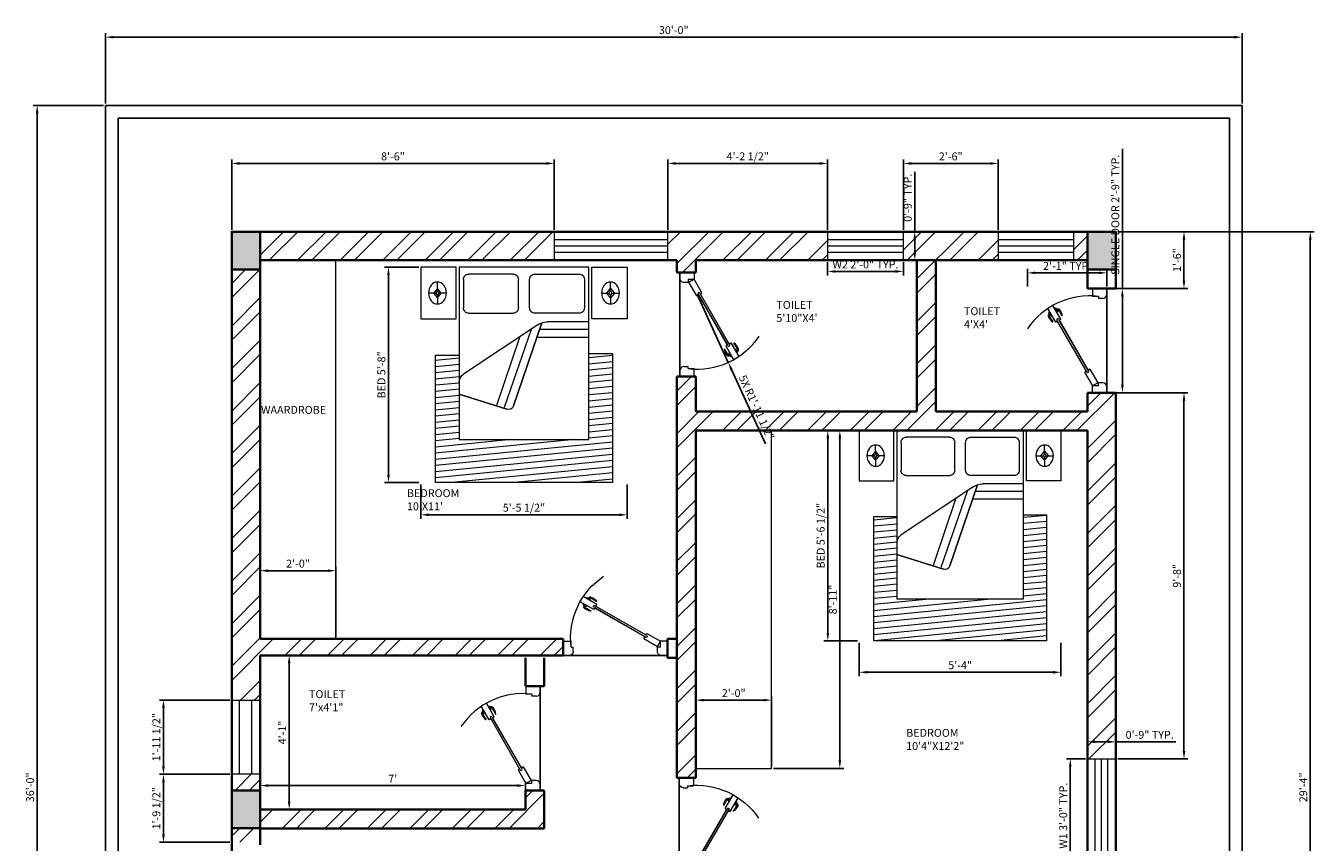
# Model space of a CAD drawing. Units: inches. Extents: x -138 to 270, y 8284 to 8764.
# Tile 10 of 10: x -138 to 270, y 8506 to 8764. Entities that reach past the tile are written whole.
import ezdxf

# ---------------------------------------------------------------- set-up
doc = ezdxf.new("R2010")
doc.units = ezdxf.units.IN
for name, color, linetype, lineweight in [('A-ANNO-DIMS', 2, 'Continuous', 18), ('A-AREA-IDEN', 7, 'Continuous', 18), ('A-FLOR-CASE', 9, 'Continuous', 18), ('C-PROP', 7, 'Continuous', 25), ('DOOR', 32, 'Continuous', 15), ('FURNITURE', 8, 'Continuous', 15), ('TEXT', 7, 'Continuous', 18), ('WALL', 8, 'Continuous', 35), ('WINDOW', 151, 'Continuous', 15)]:
    doc.layers.add(name, color=color, linetype=linetype, lineweight=lineweight)
doc.layers.add('A-COLS', color=252, linetype='Continuous', lineweight=35, true_color=0x939598)
doc.layers.add('A-WALL-PATT', color=32, linetype='Continuous', lineweight=9, true_color=0xbc761a)
doc.styles.get("Standard").update_dxf_attribs({"font": 'arial.ttf'})
doc.dimstyles.new('ISO-25', dxfattribs={"dimtxt": 2.5, "dimasz": 2.5, "dimexe": 1.25, "dimexo": 0.625, "dimtad": 1, "dimdec": 0, "dimlunit": 3, "dimtxsty": 'Standard', "dimcen": 2.5, "dimadec": 0, "dimazin": 0, "dimtfac": 1, "dimtdec": 0, "dimtmove": 0, "dimatfit": 3, "dimfxl": 1, "dimarcsym": 0})

# ---------------------------------------------------------------- blocks, each defined once
blk = doc.blocks.new('A$C188C77A6')
at = {"color": 0}
blk.add_lwpolyline([(0, 49.22), (21, 49.22, -0.086905), (23.98, 48.8), (38.29, 14.11, 0.409267), (41.68, 12.71), (65.99, 18.99), (65.99, 0), (0, 0), (0, 72.01), (65.99, 72.01), (65.99, 23.99)], format="xyb", dxfattribs=at)
for points in [[(27.5, 52.84, 0.414214), (30.17, 55.01), (30.17, 66.95, 0.414214), (27.5, 69.12), (4.89, 69.12, 0.414214), (2.22, 66.95), (2.22, 55.01, 0.414214), (4.89, 52.84)], [(38.49, 52.84, -0.414214), (35.82, 55.01), (35.82, 66.95, -0.414214), (38.49, 69.12), (61.11, 69.12, -0.414214), (63.77, 66.95), (63.77, 55.01, -0.414214), (61.11, 52.84)], [(23.98, 48.8, -0.060842), (25.88, 48.01), (63.78, 27.37, -0.250283), (65.99, 23.99), (65.99, 18.99), (41.68, 12.71, -0.409267), (38.29, 14.11)]]:
    blk.add_lwpolyline(points, format="xyb", close=True, dxfattribs=at)
for points in [[(0, 45.97), (24.66, 45.97)], [(29.33, 45.97), (43, 13.41)], [(0, 42.71), (26, 42.71)], [(35.33, 42.71), (47, 14.23)]]:
    blk.add_lwpolyline(points, dxfattribs=at)
blk = doc.blocks.new('A$C773A563A')
h = blk.add_hatch()
h.set_pattern_fill('ANSI31', color=0, scale=25, angle=135)
h.set_pattern_definition([(180, (0, 0), (-4e-16, -3.125), [])])
h.paths.add_polyline_path([(-45, -39), (-45, -92.93), (45, -92.93), (45, -39.76), (33, -39.76), (33, -51.02), (33, -56.02), (33, -75.01), (-33, -75.01), (-33, -39)])
at = {"color": 0}
for p, q in [((-44, -13.1), (-44, -9.2)), ((44, -13.1), (44, -9.2)), ((-44.65, -13.75), (-48.55, -13.75)), ((-44, -11.8), (-45.95, -13.75)), ((-45.95, -13.75), (-44, -15.7)), ((-42.05, -13.75), (-44, -11.8)), ((-44, -15.7), (-42.05, -13.75)), ((-44, -14.4), (-44, -18.3)), ((-39.45, -13.75), (-43.35, -13.75)), ((39.45, -13.75), (43.35, -13.75)), ((42.05, -13.75), (44, -11.8)), ((44, -15.7), (42.05, -13.75)), ((44, -11.8), (45.95, -13.75)), ((45.95, -13.75), (44, -15.7)), ((44, -14.4), (44, -18.3)), ((44.65, -13.75), (48.55, -13.75)), ((-33, -39), (-45, -39)), ((-45, -39), (-45, -92.93)), ((45, -39.76), (33, -39.76)), ((45, -92.93), (45, -39.76)), ((-45, -92.93), (45, -92.93))]:
    blk.add_line(p, q, dxfattribs=at)
for points in [[(-34.5, -3), (-52.5, -3), (-52.5, -24.5), (-34.5, -24.5)], [(34.5, -3), (52.5, -3), (52.5, -24.5), (34.5, -24.5)]]:
    blk.add_lwpolyline(points, close=True, dxfattribs=at)
for centre, radius in [((-44, -13.75), 4.55), ((44, -13.75), 4.55), ((-44, -13.75), 0.65), ((44, -13.75), 0.65)]:
    blk.add_circle(centre, radius, dxfattribs=at)
blk.add_blockref('A$C188C77A6', (-33, -75.01), dxfattribs=at)
blk = doc.blocks.new('A$C1A8229D7')
at = {"layer": 'DOOR'}
for p, q in [((22.38, 16.16), (26.71, 18.66)), ((23.31, 14.53), (27.64, 17.03)), ((24.39, 17.68), (25.47, 18.3)), ((24.39, 17.68), (24.54, 17.41)), ((24.56, 18), (25.1, 18.31)), ((24.56, 18), (24.66, 17.83)), ((24.56, 18), (24.56, 18)), ((24.83, 18.15), (24.83, 18.15)), ((25.1, 18.31), (25.2, 18.15)), ((25.47, 18.3), (25.62, 18.03)), ((26.72, 16.14), (26.56, 16.41)), ((27.64, 17.03), (26.71, 18.66)), ((6.56, 6.3), (22.96, 15.77)), ((23.27, 15.23), (6.87, 5.76)), ((7.14, 5.92), (23, 15.07)), ((22.69, 15.61), (22.38, 16.16)), ((23.31, 14.53), (23, 15.07)), ((23.39, 15.66), (23.39, 15.66)), ((25.64, 15.51), (25.48, 15.78)), ((25.64, 15.51), (26.72, 16.14)), ((26, 15.51), (25.91, 15.67)), ((26, 15.51), (26.54, 15.82)), ((26, 15.51), (26, 15.51)), ((26.27, 15.66), (26.27, 15.66)), ((26.54, 15.82), (26.45, 15.98)), ((0, 0), (0, 4.5)), ((0, 4.5), (2.19, 4.5)), ((6.52, 7), (2.19, 4.5)), ((2.19, 2.62), (2.19, 4.5)), ((3.12, 2.88), (2.19, 4.5)), ((7.46, 5.38), (3.12, 2.88)), ((6.45, 5.88), (6.45, 5.88)), ((6.83, 6.46), (6.52, 7)), ((7.46, 5.38), (7.14, 5.92)), ((30.5, 2.62), (30.5, 4.5)), ((33, 4.5), (30.5, 4.5)), ((33, 0), (33, 4.5)), ((2.19, 2.62), (3.12, 2.62)), ((3.12, 1.25), (3.12, 2.62)), ((29.87, 1.25), (29.87, 2.62)), ((30.5, 2.62), (29.87, 2.62)), ((0, 0), (1.87, 0)), ((33, 0), (0, 0)), ((0, 0), (33, 0)), ((33, 0), (31.12, 0))]:
    blk.add_line(p, q, dxfattribs=at)
at = {"layer": 'DOOR', "ltscale": 0.1}
blk.add_arc((6.98, 5.45), 23.69, 353.1504, 56.0415, dxfattribs=at)
at = {"layer": 'DOOR'}
for centre, radius, start, end in [((22.48, 17.15), 0.0372, 138.2373, 332.5518), ((25.46, 15.13), 3.63, 111.4546, 145.7774), ((27.78, 10.32), 8.61, 114.2033, 127.709), ((24.4, 17.99), 0.592, 22.7059, 117.5689), ((24.41, 17.91), 0.312, 30, 120), ((23.12, 15.5), 0.312, 30, 120), ((23.12, 15.5), 0.312, 300, 30), ((24.23, 14.13), 0.0372, 87.4482, 281.7627), ((20.96, 22.13), 8.61, 292.291, 305.7967), ((23.97, 17.71), 3.63, 274.2226, 308.5454), ((25.85, 15.42), 0.312, 300, 30), ((25.92, 15.37), 0.592, 302.4311, 37.2941), ((6.72, 6.03), 0.312, 120, 210), ((6.72, 6.03), 0.312, 210, 300), ((1.87, 1.25), 1.25, 270, 0), ((31.12, 1.25), 1.25, 180, 270)]:
    blk.add_arc(centre, radius, start, end, dxfattribs=at)
blk = doc.blocks.new('*D20')
at = {"layer": 'A-ANNO-DIMS', "color": 0, "lineweight": -2, "transparency": 16777216}
for p, q in [((-63.92, 8516.87), (-63.92, 8525.04)), ((20.08, 8516.87), (20.08, 8525.04)), ((-61.42, 8523.79), (17.58, 8523.79))]:
    blk.add_line(p, q, dxfattribs=at)
at = {"layer": 'A-ANNO-DIMS', "color": 0, "transparency": 16777216}
for points in [[(-61.42, 8524.21), (-61.42, 8523.37), (-63.92, 8523.79)], [(17.58, 8524.21), (17.58, 8523.37), (20.08, 8523.79)]]:
    blk.add_solid(points, dxfattribs=at)
at = {"layer": 'Defpoints', "color": 0, "transparency": 16777216}
for p in [(20.08, 8523.79), (-63.92, 8516.24), (20.08, 8516.24)]:
    blk.add_point(p, dxfattribs=at)
at = {"layer": 'A-ANNO-DIMS', "color": 0, "transparency": 16777216, "insert": (-21.92, 8525.66), "char_height": 2.5, "attachment_point": 5}
blk.add_mtext("7'", dxfattribs=at)
blk = doc.blocks.new('*D21')
at = {"layer": 'A-ANNO-DIMS', "color": 0, "lineweight": -2, "transparency": 16777216}
for p, q in [((-55.49, 8564.99), (-53.47, 8564.99)), ((-54.72, 8562.49), (-54.72, 8518.74)), ((-55.49, 8516.24), (-53.47, 8516.24))]:
    blk.add_line(p, q, dxfattribs=at)
at = {"layer": 'A-ANNO-DIMS', "color": 0, "transparency": 16777216}
for points in [[(-55.14, 8562.49), (-54.3, 8562.49), (-54.72, 8564.99)], [(-55.14, 8518.74), (-54.3, 8518.74), (-54.72, 8516.24)]]:
    blk.add_solid(points, dxfattribs=at)
at = {"layer": 'Defpoints', "color": 0, "transparency": 16777216}
for p in [(-56.11, 8564.99), (-56.11, 8516.24), (-54.72, 8516.24)]:
    blk.add_point(p, dxfattribs=at)
at = {"layer": 'A-ANNO-DIMS', "color": 0, "transparency": 16777216, "insert": (-56.6, 8540.62), "char_height": 2.5, "attachment_point": 5, "rotation": 90}
blk.add_mtext('4\'-1"', dxfattribs=at)
blk = doc.blocks.new('WINDOW-36IN')
for p, q in [((0, 6.5), (36, 6.5)), ((0, 4.5), (36, 4.5)), ((0, 2.5), (36, 2.5))]:
    blk.add_line(p, q)
blk.add_lwpolyline([(0, 0), (36, 0), (36, 9), (0, 9)], close=True)
blk = doc.blocks.new('WINDOW-24IN')
for p, q in [((0, 6.5), (24, 6.5)), ((0, 4.5), (24, 4.5)), ((0, 2.5), (24, 2.5))]:
    blk.add_line(p, q)
blk.add_lwpolyline([(0, 0), (24, 0), (24, 9), (0, 9)], close=True)
blk = doc.blocks.new('COLUMN-9X12IN')
h = blk.add_hatch(color=256)
h.dxf.hatch_style = 1
h.paths.add_polyline_path([(9, 12), (0, 12), (0, 0), (9, 0)])
blk.add_lwpolyline([(0, 0), (9, 0), (9, 12), (0, 12)], close=True)
blk = doc.blocks.new('*D31')
at = {"layer": 'A-ANNO-DIMS', "color": 0, "lineweight": -2, "transparency": 16777216}
for p, q in [((209.18, 8681.24), (209.18, 8725.45)), ((204.85, 8681.24), (210.43, 8681.24)), ((209.18, 8650.74), (209.18, 8678.74)), ((204.85, 8648.24), (210.43, 8648.24))]:
    blk.add_line(p, q, dxfattribs=at)
at = {"layer": 'A-ANNO-DIMS', "color": 0, "transparency": 16777216}
for points in [[(208.76, 8678.74), (209.59, 8678.74), (209.18, 8681.24)], [(208.76, 8650.74), (209.59, 8650.74), (209.18, 8648.24)]]:
    blk.add_solid(points, dxfattribs=at)
at = {"layer": 'Defpoints', "color": 0, "transparency": 16777216}
for p in [(204.23, 8681.24), (209.18, 8681.24), (204.23, 8648.24)]:
    blk.add_point(p, dxfattribs=at)
at = {"layer": 'A-ANNO-DIMS', "color": 0, "transparency": 16777216, "insert": (207.26, 8704.6), "char_height": 2.5, "attachment_point": 5, "rotation": 90}
blk.add_mtext('SINGLE DOOR 2\'-9" TYP.', dxfattribs=at)
blk = doc.blocks.new('*D32')
at = {"layer": 'A-ANNO-DIMS', "color": 0, "lineweight": -2, "transparency": 16777216}
for p, q in [((179.13, 8681.87), (179.13, 8687.44)), ((201.73, 8686.19), (181.63, 8686.19)), ((204.23, 8681.87), (204.23, 8687.44))]:
    blk.add_line(p, q, dxfattribs=at)
at = {"layer": 'A-ANNO-DIMS', "color": 0, "transparency": 16777216}
for points in [[(181.63, 8686.61), (181.63, 8685.78), (179.13, 8686.19)], [(201.73, 8686.61), (201.73, 8685.78), (204.23, 8686.19)]]:
    blk.add_solid(points, dxfattribs=at)
at = {"layer": 'Defpoints', "color": 0, "transparency": 16777216}
for p in [(179.13, 8686.19), (179.13, 8681.24), (204.23, 8681.24)]:
    blk.add_point(p, dxfattribs=at)
at = {"layer": 'A-ANNO-DIMS', "color": 0, "transparency": 16777216, "insert": (191.68, 8688.07), "char_height": 2.5, "attachment_point": 5}
blk.add_mtext('2\'-1" TYP.', dxfattribs=at)
blk = doc.blocks.new('*D33')
at = {"layer": 'A-ANNO-DIMS', "color": 0, "lineweight": -2, "transparency": 16777216}
for p, q in [((197.45, 8532.24), (191.43, 8532.24)), ((192.68, 8498.74), (192.68, 8529.74)), ((197.45, 8496.24), (191.43, 8496.24))]:
    blk.add_line(p, q, dxfattribs=at)
at = {"layer": 'A-ANNO-DIMS', "color": 0, "transparency": 16777216}
for points in [[(192.26, 8529.74), (193.09, 8529.74), (192.68, 8532.24)], [(192.26, 8498.74), (193.09, 8498.74), (192.68, 8496.24)]]:
    blk.add_solid(points, dxfattribs=at)
at = {"layer": 'Defpoints', "color": 0, "transparency": 16777216}
for p in [(192.68, 8532.24), (198.08, 8532.24), (198.08, 8496.24)]:
    blk.add_point(p, dxfattribs=at)
at = {"layer": 'A-ANNO-DIMS', "color": 0, "transparency": 16777216, "insert": (190.77, 8514.24), "char_height": 2.5, "attachment_point": 5, "rotation": 90}
blk.add_mtext('W1 3\'-0" TYP.', dxfattribs=at)
blk = doc.blocks.new('*D34')
at = {"layer": 'A-ANNO-DIMS', "color": 0, "lineweight": -2, "transparency": 16777216}
for p, q in [((198.08, 8532.87), (198.08, 8538.89)), ((200.58, 8537.64), (204.58, 8537.64)), ((207.08, 8532.87), (207.08, 8538.89)), ((207.08, 8537.64), (226.06, 8537.64))]:
    blk.add_line(p, q, dxfattribs=at)
at = {"layer": 'A-ANNO-DIMS', "color": 0, "transparency": 16777216}
for points in [[(200.58, 8538.06), (200.58, 8537.23), (198.08, 8537.64)], [(204.58, 8538.06), (204.58, 8537.23), (207.08, 8537.64)]]:
    blk.add_solid(points, dxfattribs=at)
at = {"layer": 'Defpoints', "color": 0, "transparency": 16777216}
for p in [(207.08, 8537.64), (198.08, 8532.24), (207.08, 8532.24)]:
    blk.add_point(p, dxfattribs=at)
at = {"layer": 'A-ANNO-DIMS', "color": 0, "transparency": 16777216, "insert": (217.82, 8539.54), "char_height": 2.5, "attachment_point": 5}
blk.add_mtext('0\'-9" TYP.', dxfattribs=at)
blk = doc.blocks.new('*D35')
at = {"layer": 'A-ANNO-DIMS', "color": 0, "lineweight": -2, "transparency": 16777216}
for p, q in [((115.81, 8689.62), (115.81, 8685.39)), ((139.81, 8689.62), (139.81, 8685.39)), ((118.31, 8686.64), (137.31, 8686.64))]:
    blk.add_line(p, q, dxfattribs=at)
at = {"layer": 'A-ANNO-DIMS', "color": 0, "transparency": 16777216}
for points in [[(118.31, 8687.06), (118.31, 8686.23), (115.81, 8686.64)], [(137.31, 8687.06), (137.31, 8686.23), (139.81, 8686.64)]]:
    blk.add_solid(points, dxfattribs=at)
at = {"layer": 'Defpoints', "color": 0, "transparency": 16777216}
for p in [(115.81, 8690.24), (139.81, 8690.24), (139.81, 8686.64)]:
    blk.add_point(p, dxfattribs=at)
at = {"layer": 'A-ANNO-DIMS', "color": 0, "transparency": 16777216, "insert": (127.81, 8688.54), "char_height": 2.5, "attachment_point": 5}
blk.add_mtext('W2 2\'-0" TYP.', dxfattribs=at)
blk = doc.blocks.new('*D36')
at = {"layer": 'A-ANNO-DIMS', "color": 0, "lineweight": -2, "transparency": 16777216}
for p, q in [((143.41, 8699.24), (143.41, 8718.23)), ((140.44, 8699.24), (144.66, 8699.24)), ((143.41, 8692.74), (143.41, 8696.74)), ((140.44, 8690.24), (144.66, 8690.24))]:
    blk.add_line(p, q, dxfattribs=at)
at = {"layer": 'A-ANNO-DIMS', "color": 0, "transparency": 16777216}
for points in [[(143, 8696.74), (143.83, 8696.74), (143.41, 8699.24)], [(143, 8692.74), (143.83, 8692.74), (143.41, 8690.24)]]:
    blk.add_solid(points, dxfattribs=at)
at = {"layer": 'Defpoints', "color": 0, "transparency": 16777216}
for p in [(139.81, 8699.24), (143.41, 8699.24), (139.81, 8690.24)]:
    blk.add_point(p, dxfattribs=at)
at = {"layer": 'A-ANNO-DIMS', "color": 0, "transparency": 16777216, "insert": (141.51, 8709.99), "char_height": 2.5, "attachment_point": 5, "rotation": 90}
blk.add_mtext('0\'-9" TYP.', dxfattribs=at)
blk = doc.blocks.new('*D37')
at = {"layer": 'A-ANNO-DIMS', "color": 0, "lineweight": -2, "transparency": 16777216}
for p, q in [((-13.67, 8687.97), (-24.52, 8687.97)), ((-23.27, 8622.29), (-23.27, 8685.47)), ((-13.67, 8619.79), (-24.52, 8619.79))]:
    blk.add_line(p, q, dxfattribs=at)
at = {"layer": 'A-ANNO-DIMS', "color": 0, "transparency": 16777216}
for points in [[(-23.69, 8685.47), (-22.86, 8685.47), (-23.27, 8687.97)], [(-23.69, 8622.29), (-22.86, 8622.29), (-23.27, 8619.79)]]:
    blk.add_solid(points, dxfattribs=at)
at = {"layer": 'Defpoints', "color": 0, "transparency": 16777216}
for p in [(-23.27, 8687.97), (-13.05, 8687.97), (-13.05, 8619.79)]:
    blk.add_point(p, dxfattribs=at)
at = {"layer": 'A-ANNO-DIMS', "color": 0, "transparency": 16777216, "insert": (-25.17, 8653.88), "char_height": 2.5, "attachment_point": 5, "rotation": 90}
blk.add_mtext('BED 5\'-8"', dxfattribs=at)
blk = doc.blocks.new('*D38')
at = {"layer": 'A-ANNO-DIMS', "color": 0, "lineweight": -2, "transparency": 16777216}
for p, q in [((-13.05, 8619.17), (-13.05, 8608.31)), ((52.34, 8619.17), (52.34, 8608.31)), ((49.84, 8609.56), (-10.55, 8609.56))]:
    blk.add_line(p, q, dxfattribs=at)
at = {"layer": 'A-ANNO-DIMS', "color": 0, "transparency": 16777216}
for points in [[(-10.55, 8609.98), (-10.55, 8609.15), (-13.05, 8609.56)], [(49.84, 8609.98), (49.84, 8609.15), (52.34, 8609.56)]]:
    blk.add_solid(points, dxfattribs=at)
at = {"layer": 'Defpoints', "color": 0, "transparency": 16777216}
for p in [(-13.05, 8619.79), (52.34, 8619.79), (-13.05, 8609.56)]:
    blk.add_point(p, dxfattribs=at)
at = {"layer": 'A-ANNO-DIMS', "color": 0, "transparency": 16777216, "insert": (19.65, 8611.48), "char_height": 2.5, "attachment_point": 5}
blk.add_mtext('5\'-5 1/2"', dxfattribs=at)
blk = doc.blocks.new('*D39')
at = {"layer": 'A-ANNO-DIMS', "color": 0, "lineweight": -2, "transparency": 16777216}
for p, q in [((125.24, 8636.24), (114.63, 8636.24)), ((115.88, 8572.17), (115.88, 8633.74)), ((125.24, 8569.67), (114.63, 8569.67))]:
    blk.add_line(p, q, dxfattribs=at)
at = {"layer": 'A-ANNO-DIMS', "color": 0, "transparency": 16777216}
for points in [[(115.46, 8633.74), (116.29, 8633.74), (115.88, 8636.24)], [(115.46, 8572.17), (116.29, 8572.17), (115.88, 8569.67)]]:
    blk.add_solid(points, dxfattribs=at)
at = {"layer": 'Defpoints', "color": 0, "transparency": 16777216}
for p in [(115.88, 8636.24), (125.86, 8636.24), (125.86, 8569.67)]:
    blk.add_point(p, dxfattribs=at)
at = {"layer": 'A-ANNO-DIMS', "color": 0, "transparency": 16777216, "insert": (113.96, 8602.96), "char_height": 2.5, "attachment_point": 5, "rotation": 90}
blk.add_mtext('BED 5\'-6 1/2"', dxfattribs=at)
blk = doc.blocks.new('*D40')
at = {"layer": 'A-ANNO-DIMS', "color": 0, "lineweight": -2, "transparency": 16777216}
for p, q in [((125.86, 8569.04), (125.86, 8558.43)), ((189.71, 8569.04), (189.71, 8558.43)), ((187.21, 8559.68), (128.36, 8559.68))]:
    blk.add_line(p, q, dxfattribs=at)
at = {"layer": 'A-ANNO-DIMS', "color": 0, "transparency": 16777216}
for points in [[(128.36, 8560.1), (128.36, 8559.26), (125.86, 8559.68)], [(187.21, 8560.1), (187.21, 8559.26), (189.71, 8559.68)]]:
    blk.add_solid(points, dxfattribs=at)
at = {"layer": 'Defpoints', "color": 0, "transparency": 16777216}
for p in [(125.86, 8569.67), (189.71, 8569.67), (125.86, 8559.68)]:
    blk.add_point(p, dxfattribs=at)
at = {"layer": 'A-ANNO-DIMS', "color": 0, "transparency": 16777216, "insert": (157.79, 8561.58), "char_height": 2.5, "attachment_point": 5}
blk.add_mtext('5\'-4"', dxfattribs=at)
blk = doc.blocks.new('*D51')
at = {"layer": 'A-ANNO-DIMS', "color": 0, "lineweight": -2, "transparency": 16777216}
for p, q in [((-112.92, 8739.87), (-112.92, 8762.11)), ((247.08, 8739.87), (247.08, 8762.11)), ((-110.42, 8760.86), (244.58, 8760.86))]:
    blk.add_line(p, q, dxfattribs=at)
at = {"layer": 'A-ANNO-DIMS', "color": 0, "transparency": 16777216}
for points in [[(-110.42, 8761.27), (-110.42, 8760.44), (-112.92, 8760.86)], [(244.58, 8761.27), (244.58, 8760.44), (247.08, 8760.86)]]:
    blk.add_solid(points, dxfattribs=at)
at = {"layer": 'Defpoints', "color": 0, "transparency": 16777216}
for p in [(247.08, 8760.86), (-112.92, 8739.24), (247.08, 8739.24)]:
    blk.add_point(p, dxfattribs=at)
at = {"layer": 'A-ANNO-DIMS', "color": 0, "transparency": 16777216, "insert": (67.08, 8762.76), "char_height": 2.5, "attachment_point": 5}
blk.add_mtext('30\'-0"', dxfattribs=at)
blk = doc.blocks.new('*D52')
at = {"layer": 'A-ANNO-DIMS', "color": 0, "lineweight": -2, "transparency": 16777216}
for p, q in [((-113.55, 8739.24), (-135.79, 8739.24)), ((-134.54, 8309.74), (-134.54, 8736.74)), ((-113.55, 8307.24), (-135.79, 8307.24))]:
    blk.add_line(p, q, dxfattribs=at)
at = {"layer": 'A-ANNO-DIMS', "color": 0, "transparency": 16777216}
for points in [[(-134.96, 8736.74), (-134.12, 8736.74), (-134.54, 8739.24)], [(-134.96, 8309.74), (-134.12, 8309.74), (-134.54, 8307.24)]]:
    blk.add_solid(points, dxfattribs=at)
at = {"layer": 'Defpoints', "color": 0, "transparency": 16777216}
for p in [(-134.54, 8739.24), (-112.92, 8739.24), (-112.92, 8307.24)]:
    blk.add_point(p, dxfattribs=at)
at = {"layer": 'A-ANNO-DIMS', "color": 0, "transparency": 16777216, "insert": (-136.44, 8523.24), "char_height": 2.5, "attachment_point": 5, "rotation": 90}
blk.add_mtext('36\'-0"', dxfattribs=at)
blk = doc.blocks.new('*D54')
at = {"layer": 'A-ANNO-DIMS', "color": 0, "lineweight": -2, "transparency": 16777216}
for p, q in [((207.7, 8699.24), (269.94, 8699.24)), ((268.69, 8349.74), (268.69, 8696.74)), ((207.7, 8347.24), (269.94, 8347.24))]:
    blk.add_line(p, q, dxfattribs=at)
at = {"layer": 'A-ANNO-DIMS', "color": 0, "transparency": 16777216}
for points in [[(268.27, 8696.74), (269.11, 8696.74), (268.69, 8699.24)], [(268.27, 8349.74), (269.11, 8349.74), (268.69, 8347.24)]]:
    blk.add_solid(points, dxfattribs=at)
at = {"layer": 'Defpoints', "color": 0, "transparency": 16777216}
for p in [(207.08, 8699.24), (268.69, 8699.24), (207.08, 8347.24)]:
    blk.add_point(p, dxfattribs=at)
at = {"layer": 'A-ANNO-DIMS', "color": 0, "transparency": 16777216, "insert": (266.79, 8523.24), "char_height": 2.5, "attachment_point": 5, "rotation": 90}
blk.add_mtext('29\'-4"', dxfattribs=at)
blk = doc.blocks.new('*D61')
at = {"layer": 'A-ANNO-DIMS', "color": 0, "lineweight": -2, "transparency": 16777216}
for p, q in [((-72.92, 8699.87), (-72.92, 8722.11)), ((-70.42, 8720.86), (26.72, 8720.86)), ((29.22, 8699.87), (29.22, 8722.11))]:
    blk.add_line(p, q, dxfattribs=at)
at = {"layer": 'A-ANNO-DIMS', "color": 0, "transparency": 16777216}
for points in [[(-70.42, 8721.27), (-70.42, 8720.44), (-72.92, 8720.86)], [(26.72, 8721.27), (26.72, 8720.44), (29.22, 8720.86)]]:
    blk.add_solid(points, dxfattribs=at)
at = {"layer": 'Defpoints', "color": 0, "transparency": 16777216}
for p in [(29.22, 8720.86), (-72.92, 8699.24), (29.22, 8699.24)]:
    blk.add_point(p, dxfattribs=at)
at = {"layer": 'A-ANNO-DIMS', "color": 0, "transparency": 16777216, "insert": (-21.85, 8722.76), "char_height": 2.5, "attachment_point": 5}
blk.add_mtext('8\'-6"', dxfattribs=at)
blk = doc.blocks.new('*D62')
at = {"layer": 'A-ANNO-DIMS', "color": 0, "lineweight": -2, "transparency": 16777216}
for p, q in [((65.22, 8699.87), (65.22, 8722.11)), ((67.72, 8720.86), (113.31, 8720.86)), ((115.81, 8699.87), (115.81, 8722.11))]:
    blk.add_line(p, q, dxfattribs=at)
at = {"layer": 'A-ANNO-DIMS', "color": 0, "transparency": 16777216}
for points in [[(67.72, 8721.27), (67.72, 8720.44), (65.22, 8720.86)], [(113.31, 8721.27), (113.31, 8720.44), (115.81, 8720.86)]]:
    blk.add_solid(points, dxfattribs=at)
at = {"layer": 'Defpoints', "color": 0, "transparency": 16777216}
for p in [(115.81, 8720.86), (65.22, 8699.24), (115.81, 8699.24)]:
    blk.add_point(p, dxfattribs=at)
at = {"layer": 'A-ANNO-DIMS', "color": 0, "transparency": 16777216, "insert": (90.52, 8722.78), "char_height": 2.5, "attachment_point": 5}
blk.add_mtext('4\'-2 1/2"', dxfattribs=at)
blk = doc.blocks.new('*D63')
at = {"layer": 'A-ANNO-DIMS', "color": 0, "lineweight": -2, "transparency": 16777216}
for p, q in [((139.81, 8699.87), (139.81, 8722.11)), ((142.31, 8720.86), (167.31, 8720.86)), ((169.81, 8699.87), (169.81, 8722.11))]:
    blk.add_line(p, q, dxfattribs=at)
at = {"layer": 'A-ANNO-DIMS', "color": 0, "transparency": 16777216}
for points in [[(142.31, 8721.27), (142.31, 8720.44), (139.81, 8720.86)], [(167.31, 8721.27), (167.31, 8720.44), (169.81, 8720.86)]]:
    blk.add_solid(points, dxfattribs=at)
at = {"layer": 'Defpoints', "color": 0, "transparency": 16777216}
for p in [(169.81, 8720.86), (139.81, 8699.24), (169.81, 8699.24)]:
    blk.add_point(p, dxfattribs=at)
at = {"layer": 'A-ANNO-DIMS', "color": 0, "transparency": 16777216, "insert": (154.81, 8722.76), "char_height": 2.5, "attachment_point": 5}
blk.add_mtext('2\'-6"', dxfattribs=at)
blk = doc.blocks.new('*D65')
at = {"layer": 'A-ANNO-DIMS', "color": 0, "lineweight": -2, "transparency": 16777216}
for p, q in [((-73.55, 8527.36), (-95.79, 8527.36)), ((-94.54, 8508.34), (-94.54, 8524.86)), ((-73.55, 8505.84), (-95.79, 8505.84))]:
    blk.add_line(p, q, dxfattribs=at)
at = {"layer": 'A-ANNO-DIMS', "color": 0, "transparency": 16777216}
for points in [[(-94.96, 8524.86), (-94.12, 8524.86), (-94.54, 8527.36)], [(-94.96, 8508.34), (-94.12, 8508.34), (-94.54, 8505.84)]]:
    blk.add_solid(points, dxfattribs=at)
at = {"layer": 'Defpoints', "color": 0, "transparency": 16777216}
for p in [(-94.54, 8527.36), (-72.92, 8527.36), (-72.92, 8505.84)]:
    blk.add_point(p, dxfattribs=at)
at = {"layer": 'A-ANNO-DIMS', "color": 0, "transparency": 16777216, "insert": (-96.46, 8516.6), "char_height": 2.5, "attachment_point": 5, "rotation": 90}
blk.add_mtext('1\'-9 1/2"', dxfattribs=at)
blk = doc.blocks.new('*D66')
at = {"layer": 'A-ANNO-DIMS', "color": 0, "lineweight": -2, "transparency": 16777216}
for p, q in [((-73.55, 8550.86), (-95.79, 8550.86)), ((-94.54, 8529.86), (-94.54, 8548.36)), ((-73.55, 8527.36), (-95.79, 8527.36))]:
    blk.add_line(p, q, dxfattribs=at)
at = {"layer": 'A-ANNO-DIMS', "color": 0, "transparency": 16777216}
for points in [[(-94.96, 8548.36), (-94.12, 8548.36), (-94.54, 8550.86)], [(-94.96, 8529.86), (-94.12, 8529.86), (-94.54, 8527.36)]]:
    blk.add_solid(points, dxfattribs=at)
at = {"layer": 'Defpoints', "color": 0, "transparency": 16777216}
for p in [(-94.54, 8550.86), (-72.92, 8550.86), (-72.92, 8527.36)]:
    blk.add_point(p, dxfattribs=at)
at = {"layer": 'A-ANNO-DIMS', "color": 0, "transparency": 16777216, "insert": (-96.46, 8539.11), "char_height": 2.5, "attachment_point": 5, "rotation": 90}
blk.add_mtext('1\'-11 1/2"', dxfattribs=at)
blk = doc.blocks.new('*D68')
at = {"layer": 'A-ANNO-DIMS', "color": 0, "lineweight": -2, "transparency": 16777216}
for p, q in [((207.7, 8699.24), (229.94, 8699.24)), ((228.69, 8696.74), (228.69, 8683.74)), ((207.7, 8681.24), (229.94, 8681.24))]:
    blk.add_line(p, q, dxfattribs=at)
at = {"layer": 'A-ANNO-DIMS', "color": 0, "transparency": 16777216}
for points in [[(228.27, 8696.74), (229.11, 8696.74), (228.69, 8699.24)], [(228.27, 8683.74), (229.11, 8683.74), (228.69, 8681.24)]]:
    blk.add_solid(points, dxfattribs=at)
at = {"layer": 'Defpoints', "color": 0, "transparency": 16777216}
for p in [(207.08, 8699.24), (207.08, 8681.24), (228.69, 8681.24)]:
    blk.add_point(p, dxfattribs=at)
at = {"layer": 'A-ANNO-DIMS', "color": 0, "transparency": 16777216, "insert": (226.79, 8690.24), "char_height": 2.5, "attachment_point": 5, "rotation": 90}
blk.add_mtext('1\'-6"', dxfattribs=at)
blk = doc.blocks.new('*D69')
at = {"layer": 'A-ANNO-DIMS', "color": 0, "lineweight": -2, "transparency": 16777216}
for p, q in [((207.7, 8648.24), (229.94, 8648.24)), ((228.69, 8645.74), (228.69, 8534.74)), ((207.7, 8532.24), (229.94, 8532.24))]:
    blk.add_line(p, q, dxfattribs=at)
at = {"layer": 'A-ANNO-DIMS', "color": 0, "transparency": 16777216}
for points in [[(228.27, 8645.74), (229.11, 8645.74), (228.69, 8648.24)], [(228.27, 8534.74), (229.11, 8534.74), (228.69, 8532.24)]]:
    blk.add_solid(points, dxfattribs=at)
at = {"layer": 'Defpoints', "color": 0, "transparency": 16777216}
for p in [(207.08, 8648.24), (207.08, 8532.24), (228.69, 8532.24)]:
    blk.add_point(p, dxfattribs=at)
at = {"layer": 'A-ANNO-DIMS', "color": 0, "transparency": 16777216, "insert": (226.79, 8590.24), "char_height": 2.5, "attachment_point": 5, "rotation": 90}
blk.add_mtext('9\'-8"', dxfattribs=at)
blk = doc.blocks.new('*D70')
at = {"layer": 'A-ANNO-DIMS', "color": 0, "lineweight": -2, "transparency": 16777216}
for p, q in [((-63.92, 8570.87), (-63.92, 8593.11)), ((-61.42, 8591.86), (-42.42, 8591.86)), ((-39.92, 8570.87), (-39.92, 8593.11))]:
    blk.add_line(p, q, dxfattribs=at)
at = {"layer": 'A-ANNO-DIMS', "color": 0, "transparency": 16777216}
for points in [[(-61.42, 8592.27), (-61.42, 8591.44), (-63.92, 8591.86)], [(-42.42, 8592.27), (-42.42, 8591.44), (-39.92, 8591.86)]]:
    blk.add_solid(points, dxfattribs=at)
at = {"layer": 'Defpoints', "color": 0, "transparency": 16777216}
for p in [(-39.92, 8591.86), (-63.92, 8570.24), (-39.92, 8570.24)]:
    blk.add_point(p, dxfattribs=at)
at = {"layer": 'A-ANNO-DIMS', "color": 0, "transparency": 16777216, "insert": (-51.92, 8593.76), "char_height": 2.5, "attachment_point": 5}
blk.add_mtext('2\'-0"', dxfattribs=at)
blk = doc.blocks.new('*D71')
at = {"layer": 'A-ANNO-DIMS', "color": 0, "lineweight": -2, "transparency": 16777216}
for p, q in [((74.08, 8529.87), (74.08, 8552.11)), ((76.58, 8550.86), (95.58, 8550.86)), ((98.08, 8529.87), (98.08, 8552.11))]:
    blk.add_line(p, q, dxfattribs=at)
at = {"layer": 'A-ANNO-DIMS', "color": 0, "transparency": 16777216}
for points in [[(76.58, 8551.27), (76.58, 8550.44), (74.08, 8550.86)], [(95.58, 8551.27), (95.58, 8550.44), (98.08, 8550.86)]]:
    blk.add_solid(points, dxfattribs=at)
at = {"layer": 'Defpoints', "color": 0, "transparency": 16777216}
for p in [(98.08, 8550.86), (74.08, 8529.24), (98.08, 8529.24)]:
    blk.add_point(p, dxfattribs=at)
at = {"layer": 'A-ANNO-DIMS', "color": 0, "transparency": 16777216, "insert": (86.08, 8552.76), "char_height": 2.5, "attachment_point": 5}
blk.add_mtext('2\'-0"', dxfattribs=at)
blk = doc.blocks.new('*D72')
at = {"layer": 'A-ANNO-DIMS', "color": 0, "lineweight": -2, "transparency": 16777216}
for p, q in [((98.7, 8636.24), (120.94, 8636.24)), ((119.69, 8633.74), (119.69, 8531.74)), ((98.7, 8529.24), (120.94, 8529.24))]:
    blk.add_line(p, q, dxfattribs=at)
at = {"layer": 'A-ANNO-DIMS', "color": 0, "transparency": 16777216}
for points in [[(119.27, 8633.74), (120.11, 8633.74), (119.69, 8636.24)], [(119.27, 8531.74), (120.11, 8531.74), (119.69, 8529.24)]]:
    blk.add_solid(points, dxfattribs=at)
at = {"layer": 'Defpoints', "color": 0, "transparency": 16777216}
for p in [(98.08, 8636.24), (98.08, 8529.24), (119.69, 8529.24)]:
    blk.add_point(p, dxfattribs=at)
at = {"layer": 'A-ANNO-DIMS', "color": 0, "transparency": 16777216, "insert": (117.79, 8582.74), "char_height": 2.5, "attachment_point": 5, "rotation": 90}
blk.add_mtext('8\'-11"', dxfattribs=at)
blk = doc.blocks.new('*D77')
at = {"layer": 'A-ANNO-DIMS', "color": 0, "lineweight": -2, "transparency": 16777216}
for p, q in [((74.47, 8679.37), (84.33, 8657.84)), ((96.16, 8631.99), (85.37, 8655.56))]:
    blk.add_line(p, q, dxfattribs=at)
at = {"layer": 'A-ANNO-DIMS', "color": 0, "transparency": 16777216}
blk.add_solid([(85.75, 8655.74), (84.99, 8655.39), (84.33, 8657.84)], dxfattribs=at)
at = {"layer": 'Defpoints', "color": 0, "transparency": 16777216}
for p in [(74.47, 8679.37), (84.33, 8657.84)]:
    blk.add_point(p, dxfattribs=at)
at = {"layer": 'A-ANNO-DIMS', "color": 0, "transparency": 16777216, "insert": (93.03, 8643.44), "char_height": 2.5, "attachment_point": 5, "rotation": 294.5954}
blk.add_mtext('5X R1\'-11 1/2"', dxfattribs=at)

msp = doc.modelspace()

# ---------------------------------------------------------------- hatches: boundary and pattern name
at = {"layer": 'A-WALL-PATT'}
h = msp.add_hatch(dxfattribs=at)
h.set_pattern_fill('ANSI32', color=256)
h.paths.add_polyline_path([(29.22, 8699.24), (-63.92, 8699.24), (-63.92, 8690.24), (29.22, 8690.24)])
h.paths.add_polyline_path([(-63.92, 8687.24), (-72.92, 8687.24), (-72.92, 8550.86), (-63.92, 8550.86), (-63.92, 8564.99), (32.08, 8564.99), (32.04, 8570.24), (-63.92, 8570.24)])
h = msp.add_hatch(dxfattribs=at)
h.set_pattern_fill('ANSI32', color=256)
h.paths.add_polyline_path([(115.81, 8699.24), (65.22, 8699.24), (65.22, 8690.24), (68.08, 8690.24), (68.08, 8686.36), (69.02, 8686.36), (69.02, 8686.36), (73.52, 8686.36), (74.08, 8686.36), (74.08, 8690.24), (115.81, 8690.24)])
h.paths.add_polyline_path([(169.81, 8699.24), (139.81, 8699.24), (139.81, 8690.24), (169.81, 8690.24)])
h.paths.add_polyline_path([(198.08, 8699.24), (193.81, 8699.24), (193.81, 8690.24), (198.08, 8690.24)])
h.paths.add_polyline_path([(207.08, 8648.24), (204.23, 8648.24), (204.23, 8648.24), (199.73, 8648.24), (198.08, 8648.24), (198.08, 8642.24), (150.08, 8642.24), (150.08, 8690.24), (144.08, 8690.24), (144.08, 8642.24), (74.08, 8642.24), (74.08, 8653.36), (68.08, 8653.36), (68.08, 8526.24), (68.83, 8526.24), (74.08, 8526.24), (74.08, 8630.24), (74.08, 8636.24), (98.08, 8636.24), (150.08, 8636.24), (198.08, 8636.24), (198.08, 8630.24), (198.08, 8532.24), (207.08, 8532.24)])
h.paths.add_polyline_path([(207.08, 8484.24), (198.08, 8484.24), (198.08, 8433.43), (207.08, 8433.43)])
h.paths.add_polyline_path([(198.08, 8490.24), (80.08, 8490.24), (80.08, 8484.24), (198.08, 8484.24)])
h.paths.add_polyline_path([(207.08, 8397.43), (198.08, 8397.43), (198.08, 8359.27), (207.08, 8359.27)])
h.paths.add_polyline_path([(198.08, 8356.24), (186.08, 8356.24), (186.08, 8347.24), (198.08, 8347.24)])
h.paths.add_polyline_path([(138.08, 8356.24), (128.38, 8356.24), (128.38, 8347.24), (138.08, 8347.24)])
h.paths.add_polyline_path([(92.38, 8356.24), (86.08, 8356.24), (86.08, 8347.24), (92.38, 8347.24)])
h = msp.add_hatch(dxfattribs=at)
h.set_pattern_fill('ANSI32', color=256)
h.paths.add_polyline_path([(-23.4, 8356.24), (-63.92, 8356.24), (-63.92, 8347.24), (-23.4, 8347.24)])
h.paths.add_polyline_path([(-63.92, 8469.84), (-72.92, 8469.84), (-72.92, 8359.24), (-63.92, 8359.24)])
h.paths.add_polyline_path([(-63.92, 8510.27), (-72.92, 8510.27), (-72.92, 8505.84), (-63.92, 8505.84)])
h.paths.add_polyline_path([(-63.92, 8527.36), (-72.92, 8527.36), (-72.92, 8522.27), (-63.92, 8522.27)])
h.paths.add_polyline_path([(26.08, 8522.24), (24.78, 8522.24), (24.78, 8522.24), (20.08, 8522.24), (20.08, 8516.24), (-63.92, 8516.24), (-63.92, 8510.24), (26.08, 8510.24)])
h.paths.add_polyline_path([(34.02, 8398.24), (34.02, 8404.24), (26.08, 8404.24), (26.08, 8356.24), (12.6, 8356.24), (12.6, 8347.24), (37.77, 8347.24), (37.77, 8356.24), (32.08, 8356.24), (32.08, 8398.24)])
h.paths.add_polyline_path([(67.02, 8404.24), (67.02, 8398.24), (68.08, 8398.24), (68.08, 8356.24), (61.77, 8356.24), (61.77, 8347.24), (74.08, 8347.24), (74.08, 8356.24), (74.08, 8356.24), (74.08, 8449.75), (68.08, 8449.75), (68.08, 8404.24)])

# ---------------------------------------------------------------- linework, layer by layer
at = {"layer": 'A-FLOR-CASE'}
for points in [[(-63.92, 8570.24), (-39.92, 8570.24), (-39.92, 8690.24), (-63.92, 8690.24)], [(74.08, 8529.24), (98.08, 8529.24), (98.08, 8636.24), (74.08, 8636.24)]]:
    msp.add_lwpolyline(points, close=True, dxfattribs=at)
at = {"layer": 'C-PROP'}
for p, q in [((-112.92, 8739.24), (247.08, 8739.24)), ((-112.92, 8739.24), (-112.92, 8307.24)), ((247.08, 8739.24), (247.08, 8307.24)), ((-108.92, 8735.24), (243.08, 8735.24)), ((-108.92, 8735.24), (-108.92, 8311.24)), ((243.08, 8735.24), (243.08, 8311.24))]:
    msp.add_line(p, q, dxfattribs=at)
at = {"layer": 'WALL'}
for p, q in [((-72.92, 8699.24), (207.08, 8699.24)), ((-72.92, 8699.24), (-72.92, 8528.24)), ((207.08, 8699.24), (207.08, 8681.24)), ((-63.92, 8690.24), (-63.92, 8570.24)), ((68.08, 8690.24), (-63.92, 8690.24)), ((68.08, 8690.24), (68.08, 8686.36)), ((74.08, 8690.24), (198.08, 8690.24)), ((74.08, 8690.24), (74.08, 8686.36)), ((144.08, 8690.24), (144.08, 8642.24)), ((150.08, 8690.24), (150.08, 8642.24)), ((198.08, 8690.24), (198.08, 8681.24)), ((74.08, 8686.36), (68.08, 8686.36)), ((207.08, 8681.24), (198.08, 8681.24)), ((68.08, 8653.36), (74.08, 8653.36)), ((68.08, 8653.36), (68.08, 8526.24)), ((74.08, 8642.24), (74.08, 8653.36)), ((198.08, 8642.24), (198.08, 8648.24)), ((198.08, 8648.24), (207.08, 8648.24)), ((198.08, 8648.24), (198.08, 8642.24)), ((207.08, 8648.24), (207.08, 8347.24)), ((74.08, 8642.24), (144.08, 8642.24)), ((150.08, 8642.24), (198.08, 8642.24)), ((74.08, 8636.24), (150.08, 8636.24)), ((74.08, 8636.24), (74.08, 8630.24)), ((150.08, 8636.24), (198.08, 8636.24)), ((198.08, 8636.24), (198.08, 8630.24)), ((74.08, 8630.24), (74.08, 8526.24)), ((198.08, 8630.24), (198.08, 8490.24)), ((-63.92, 8570.24), (32.04, 8570.24)), ((32.08, 8564.99), (32.04, 8570.24)), ((65.08, 8570.24), (68.08, 8570.24)), ((65.08, 8564.24), (65.08, 8570.24)), ((-63.92, 8564.99), (32.08, 8564.99)), ((-63.92, 8564.99), (-63.92, 8504.99)), ((20.08, 8564.24), (20.08, 8555.24)), ((26.08, 8564.24), (26.08, 8555.24)), ((65.08, 8564.24), (68.08, 8564.24)), ((20.08, 8555.24), (26.08, 8555.24)), ((-72.92, 8528.24), (-72.92, 8347.24)), ((74.08, 8526.24), (68.08, 8526.24)), ((20.08, 8516.24), (20.08, 8522.24)), ((20.08, 8522.24), (26.08, 8522.24)), ((20.08, 8522.24), (20.08, 8516.24)), ((26.08, 8522.24), (26.08, 8510.24)), ((-63.92, 8516.24), (20.08, 8516.24)), ((-63.92, 8510.24), (26.08, 8510.24))]:
    msp.add_line(p, q, dxfattribs=at)
at = {"layer": 'WINDOW'}
for points in [[(-72.92, 8550.86), (-63.92, 8550.86), (-63.92, 8527.36), (-72.92, 8527.36)], [(-70.48, 8550.86), (-66.65, 8550.86), (-66.65, 8527.36), (-70.48, 8527.36)]]:
    msp.add_lwpolyline(points, close=True, dxfattribs=at)

# ---------------------------------------------------------------- block references
at = {"layer": 'A-COLS'}
for p in [(-72.92, 8687.24), (198.08, 8687.24), (-72.92, 8510.27)]:
    msp.add_blockref('COLUMN-9X12IN', p, dxfattribs=at)
at = {"layer": 'DOOR'}
for p, rotation in [((69.02, 8686.36), 270), ((204.23, 8648.24), 90), ((24.78, 8522.24), 90)]:
    msp.add_blockref('A$C1A8229D7', p, dxfattribs=dict(at, rotation=rotation))
at = {"layer": 'DOOR', "xscale": -1}
for p, rotation in [((65.08, 8564.99), 0.001681390743995), ((68.83, 8493.24), 270)]:
    msp.add_blockref('A$C1A8229D7', p, dxfattribs=dict(at, rotation=rotation))
at = {"layer": 'FURNITURE', "extrusion": (0, 0, -1)}
for p, xscale, yscale, zscale in [((-19.65, 8690.24), 0.6227952179853853, 0.7581257236178822, -0.6227952179854009), ((-157.79, 8638.46), 0.6081543529692283, 0.7403034666958224, -0.6081543529692434)]:
    msp.add_blockref('A$C773A563A', p, dxfattribs=dict(at, xscale=xscale, yscale=yscale, zscale=zscale))
at = {"layer": 'WINDOW'}
for name, p in [('WINDOW-36IN', (29.22, 8690.24)), ('WINDOW-24IN', (115.81, 8690.24)), ('WINDOW-24IN', (169.81, 8690.24))]:
    msp.add_blockref(name, p, dxfattribs=at)
at = {"layer": 'WINDOW', "extrusion": (0, 0, -1), "zscale": -1, "rotation": 89.99999999999204}
msp.add_blockref('WINDOW-36IN', (-198.08, 8496.24), dxfattribs=at)

# ---------------------------------------------------------------- texts
at = {"layer": 'A-AREA-IDEN', "char_height": 2.5, "attachment_point": 1}
for s, width, insert in [('TOILET\\P5\'10"X4\'', 18.3346, (99.58, 8677.3)), ("TOILET\\P4'X4'", 17.2301, (159, 8675.31)), ("BEDROOM\\P10'X11'", 38.0764, (-17.41, 8617.66)), ('TOILET \\P7\'x4\'1"', 40.6832, (-48.44, 8553.99)), ('BEDROOM\\P10\'4"X12\'2"', 38.0764, (140.7, 8541.74))]:
    msp.add_mtext_dynamic_manual_height_columns(s, width=width, gutter_width=12.5, heights=[0], dxfattribs=dict(at, insert=insert))
at = {"layer": 'TEXT', "insert": (-63.62, 8644.05), "char_height": 2.5, "attachment_point": 1}
msp.add_mtext_dynamic_manual_height_columns('WAARDROBE', width=7.3004, gutter_width=12.5, heights=[0], dxfattribs=at)

# ---------------------------------------------------------------- dimensions: what is measured, and where the dimension line sits
at = {"layer": 'A-ANNO-DIMS'}
for base, p1, p2, picture, middle in [((247.08, 8760.86), (-112.92, 8739.24), (247.08, 8739.24), '*D51', (67.08, 8762.76)), ((29.22, 8720.86), (-72.92, 8699.24), (29.22, 8699.24), '*D61', (-21.85, 8722.76)), ((169.81, 8720.86), (139.81, 8699.24), (169.81, 8699.24), '*D63', (154.81, 8722.76)), ((-39.92, 8591.86), (-63.92, 8570.24), (-39.92, 8570.24), '*D70', (-51.92, 8593.76)), ((98.08, 8550.86), (74.08, 8529.24), (98.08, 8529.24), '*D71', (86.08, 8552.76))]:
    dim = msp.add_linear_dim(base=base, p1=p1, p2=p2, dimstyle='ISO-25', override={"dimdec": 1, "dimlfac": 1, "dimrnd": 0, "dimzin": 1, "dimdsep": 46, "dimlunit": 4, "dimfrac": 2}, dxfattribs=at)
    dim.commit()
    dim.dimension.update_dxf_attribs({"geometry": picture, "text_midpoint": middle})
for base, p1, p2, angle, picture, middle in [((-134.54, 8739.24), (-112.92, 8307.24), (-112.92, 8739.24), 90, '*D52', (-136.44, 8523.24)), ((115.81, 8720.86), (65.22, 8699.24), (115.81, 8699.24), 0, '*D62', (90.52, 8722.78)), ((268.69, 8699.24), (207.08, 8347.24), (207.08, 8699.24), 90, '*D54', (266.79, 8523.24)), ((228.69, 8681.24), (207.08, 8699.24), (207.08, 8681.24), 270, '*D68', (226.79, 8690.24)), ((228.69, 8532.24), (207.08, 8648.24), (207.08, 8532.24), 270, '*D69', (226.79, 8590.24)), ((119.69, 8529.24), (98.08, 8636.24), (98.08, 8529.24), 270, '*D72', (117.79, 8582.74)), ((-13.05, 8609.56), (52.34, 8619.79), (-13.05, 8619.79), 180, '*D38', (19.65, 8611.48)), ((125.8619, 8559.6813), (189.7144, 8569.6676), (125.8619, 8569.6676), 180, '*D40', (157.7881, 8561.5776)), ((-94.54, 8550.86), (-72.92, 8527.36), (-72.92, 8550.86), 90, '*D66', (-96.46, 8539.11)), ((-94.54, 8527.36), (-72.92, 8505.84), (-72.92, 8527.36), 90, '*D65', (-96.46, 8516.6))]:
    dim = msp.add_linear_dim(base=base, p1=p1, p2=p2, angle=angle, dimstyle='ISO-25', override={"dimdec": 1, "dimlfac": 1, "dimrnd": 0, "dimzin": 1, "dimdsep": 46, "dimlunit": 4, "dimfrac": 2}, dxfattribs=at)
    dim.commit()
    dim.dimension.update_dxf_attribs({"geometry": picture, "text_midpoint": middle})
for base, p1, p2, angle, text, picture, middle in [((209.18, 8681.24), (204.23, 8648.24), (204.23, 8681.24), 90, 'SINGLE DOOR <> TYP.', '*D31', (207.26, 8704.6)), ((143.41, 8699.24), (139.81, 8690.24), (139.81, 8699.24), 90, '<> TYP.', '*D36', (141.51, 8709.99)), ((179.13, 8686.19), (204.23, 8681.24), (179.13, 8681.24), 180, '<> TYP.', '*D32', (191.68, 8688.07)), ((-23.27, 8687.97), (-13.05, 8619.79), (-13.05, 8687.97), 90, 'BED <>', '*D37', (-25.17, 8653.88)), ((115.88, 8636.24), (125.86, 8569.67), (125.86, 8636.24), 90, 'BED <>', '*D39', (113.96, 8602.96)), ((207.08, 8537.64), (198.08, 8532.24), (207.08, 8532.24), 0, '<> TYP.', '*D34', (217.82, 8539.54)), ((192.68, 8532.24), (198.08, 8496.24), (198.08, 8532.24), 90, 'W1 <> TYP.', '*D33', (190.77, 8514.24))]:
    dim = msp.add_linear_dim(base=base, p1=p1, p2=p2, angle=angle, text=text, dimstyle='ISO-25', override={"dimdec": 1, "dimlfac": 1, "dimrnd": 0, "dimzin": 1, "dimdsep": 46, "dimlunit": 4, "dimfrac": 2}, dxfattribs=at)
    dim.commit()
    dim.dimension.update_dxf_attribs({"geometry": picture, "text_midpoint": middle})
dim = msp.add_linear_dim(base=(139.81, 8686.64), p1=(115.81, 8690.24), p2=(139.81, 8690.24), text='W2 <> TYP.', dimstyle='ISO-25', override={"dimdec": 1, "dimlfac": 1, "dimrnd": 0, "dimzin": 1, "dimdsep": 46, "dimlunit": 4, "dimfrac": 2}, dxfattribs=at)
dim.commit()
dim.dimension.update_dxf_attribs({"geometry": '*D35', "text_midpoint": (127.81, 8688.54)})
dim = msp.add_radius_dim(center=(74.47, 8679.37), mpoint=(84.33, 8657.84), text='5X <>', dimstyle='ISO-25', override={"dimdec": 1, "dimlfac": 1, "dimrnd": 0, "dimzin": 1, "dimdsep": 46, "dimlunit": 4, "dimfrac": 2}, dxfattribs=at)
dim.commit()
dim.dimension.update_dxf_attribs({"geometry": '*D77', "text_midpoint": (93.03, 8643.44)})
for p1, p2, distance, picture, middle in [((-56.11, 8564.99), (-56.11, 8516.24), 1.39, '*D21', (-56.6, 8540.62)), ((-63.92, 8516.24), (20.08, 8516.24), 7.55, '*D20', (-21.92, 8525.66))]:
    dim = msp.add_aligned_dim(p1=p1, p2=p2, distance=distance, dimstyle='ISO-25', override={"dimclrd": 0, "dimclre": 0, "dimclrt": 0}, dxfattribs=at)
    dim.commit()
    dim.dimension.update_dxf_attribs({"geometry": picture, "text_midpoint": middle})

doc.saveas('drawing.dxf')
